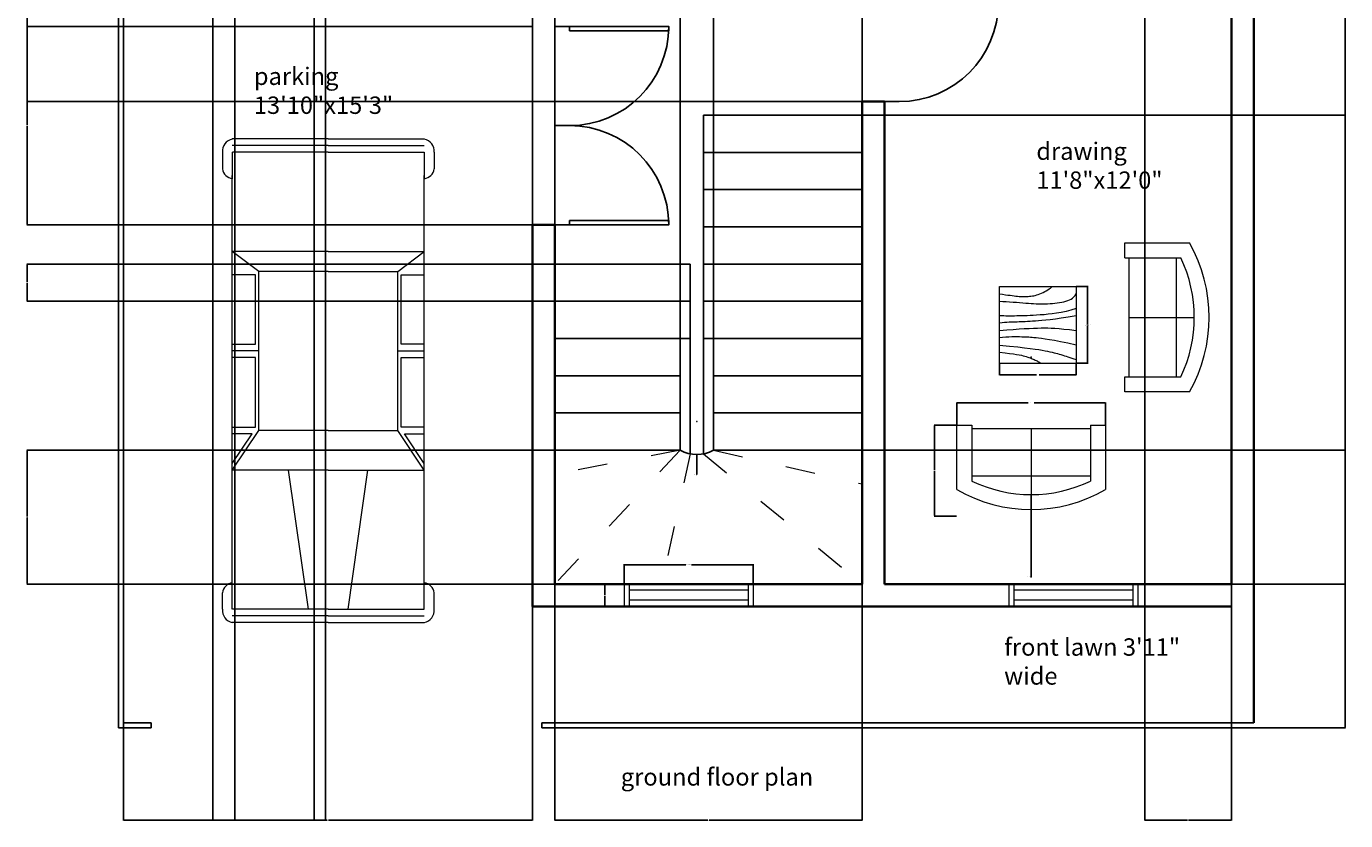
# Model space of a CAD drawing. Units: inches. Extents: x 1801 to 2333, y 478 to 1258.
# Tile 1 of 3: x 1801 to 2333, y 478 to 798. Entities that reach past the tile are written whole.
import ezdxf

# ---------------------------------------------------------------- set-up
doc = ezdxf.new("R2010")
doc.units = ezdxf.units.IN
doc.header["$MEASUREMENT"] = 0
doc.linetypes.add('ACAD_ISO03W100', pattern=[30, 12, -18])
for name, color, linetype, lineweight in [('A-ANNO-DIMS', 2, 'Continuous', 18), ('A-ANNO-TEXT', 7, 'Continuous', 25), ('A-AREA-IDEN', 7, 'Continuous', 18), ('A-DOOR', 4, 'Continuous', 25), ('A-FLOR-STRS', 7, 'Continuous', 25), ('A-FLOR-STRS-OVHD', 7, 'ACAD_ISO03W100', 18), ('A-FURN', 8, 'Continuous', 18), ('A-GLAZ', 4, 'Continuous', 18), ('A-WALL', 7, 'Continuous', 35), ('C-PKNG-VEHI', 8, 'Continuous', 13), ('C-PROP', 3, 'Continuous', 25)]:
    doc.layers.add(name, color=color, linetype=linetype, lineweight=lineweight)
doc.styles.get("Standard").update_dxf_attribs({"font": 'arial.ttf'})
doc.dimstyles.get("Standard").update_dxf_attribs({"dimtxt": 0.18, "dimasz": 0.18, "dimexe": 0.18, "dimexo": 0.0625, "dimgap": 0.09, "dimtad": 0, "dimtih": 1, "dimtoh": 1, "dimdec": 0, "dimzin": 0, "dimdsep": 46, "dimlunit": 3, "dimtxsty": 'Standard', "dimcen": 0.09, "dimadec": 0, "dimazin": 0, "dimtfac": 1, "dimtdec": 0, "dimtofl": 0, "dimtmove": 0, "dimatfit": 3, "dimfxl": 1, "dimtolj": 1, "dimtzin": 0, "dimarcsym": 0})

# ---------------------------------------------------------------- blocks, each defined once
blk = doc.blocks.new('*U2')
for p, q in [((0, 0), (0, -6)), ((40, 0), (40, -6))]:
    blk.add_line(p, q)
blk.add_lwpolyline([(0, 0), (0, 40), (1.75, 40), (1.75, 0)], close=True)
blk.add_arc((0, 0), 40, 0, 90)
blk = doc.blocks.new('*U4')
for p, q in [((0.1, -0.41), (0.1, 38.35)), ((2.77, -0.41), (2.77, 38.31)), ((5.44, 42.31), (12.12, 42.31)), ((5.44, -0.41), (5.44, 38.24)), ((5.45, 38.31), (16.12, 38.31)), ((16.12, 38.31), (180.34, 38.31)), ((61.52, -0.41), (61.52, 38.31)), ((61.52, 38.31), (77.54, 27.62)), ((64.19, 38.31), (76.2, 30.29)), ((76.2, 30.29), (76.2, 38.31)), ((78.87, 38.31), (78.87, 28.96)), ((106.91, 28.96), (106.91, 38.31)), ((109.58, 27.62), (109.58, 38.31)), ((112.25, 38.31), (112.25, 28.96)), ((140.29, 28.96), (140.29, 38.31)), ((141.62, 27.62), (149.64, 38.31)), ((149.64, -0.41), (149.64, 38.31)), ((189.69, 38.31), (179.01, 38.31)), ((189.69, 42.31), (183.01, 42.31)), ((189.69, -0.41), (189.69, 38.24)), ((192.36, -0.41), (192.36, 38.31)), ((195.03, -0.41), (195.03, 38.35)), ((77.54, 27.62), (141.62, 27.62)), ((77.54, -0.41), (77.54, 27.62)), ((78.87, 28.96), (106.91, 28.96)), ((112.25, 28.96), (140.29, 28.96)), ((141.62, -0.41), (141.62, 27.62)), ((5.44, 7.6), (61.52, 15.61)), ((0.1, -0.42), (0.1, -39.18)), ((2.77, -0.41), (2.77, -39.13)), ((5.44, -0.42), (5.44, -39.07)), ((61.52, -0.41), (61.52, -39.13)), ((77.54, -0.41), (77.54, -28.45)), ((141.62, -0.41), (141.62, -28.45)), ((149.64, -0.41), (149.64, -39.13)), ((189.69, -0.42), (189.69, -39.07)), ((192.36, -0.41), (192.36, -39.13)), ((195.03, -0.42), (195.03, -39.18)), ((5.44, -8.42), (61.52, -16.43)), ((61.52, -39.13), (77.54, -28.45)), ((64.19, -39.13), (76.2, -31.12)), ((76.2, -31.12), (76.2, -39.13)), ((77.54, -28.45), (141.62, -28.45)), ((78.87, -39.13), (78.87, -29.79)), ((78.87, -29.79), (106.91, -29.79)), ((106.91, -29.79), (106.91, -39.13)), ((109.58, -28.45), (109.58, -39.13)), ((112.25, -29.79), (140.29, -29.79)), ((112.25, -39.13), (112.25, -29.79)), ((140.29, -29.79), (140.29, -39.13)), ((141.62, -28.45), (149.64, -39.13)), ((5.45, -39.13), (16.12, -39.13)), ((16.12, -39.13), (180.34, -39.13)), ((189.69, -39.13), (179.01, -39.13)), ((5.44, -43.14), (12.12, -43.14)), ((189.69, -43.14), (183.01, -43.14))]:
    blk.add_line(p, q)
for centre, radius, start, end in [((5.06, 37.26), 5.06, 85.6455, 168.0943), ((11.45, 37.64), 4.72, 8.1301, 81.87), ((183.68, 37.64), 4.72, 98.13, 171.8699), ((190.07, 37.26), 5.06, 11.9057, 94.3545), ((5.06, -38.09), 5.06, 191.9057, 274.3545), ((11.45, -38.46), 4.72, 278.13, 351.8699), ((183.68, -38.46), 4.72, 188.1301, 261.87), ((190.07, -38.09), 5.06, 265.6455, 348.0943)]:
    blk.add_arc(centre, radius, start, end)
blk = doc.blocks.new('Sofa - Roundback Loveseat 5 ft.')
for p, q in [((0, -32.44198), (0, -5.99998)), ((-24, -33.99998), (-24, -11.46958)), ((-23.9998, -13.38178), (23.99986, -13.38178)), ((24.00004, -33.99998), (24.00004, -11.46958)), ((-24, -32.44198), (24.00004, -32.44198))]:
    blk.add_line(p, q)
for points in [[(-24, -33.99998), (-30, -33.99998), (-30, -7.99998)], [(30.00004, -7.99998), (30.00004, -33.99998), (24.00004, -33.99998)]]:
    blk.add_lwpolyline(points)
for centre, radius, start, end in [((0, -60.24998), 60.24998, 60.13715, 119.8628), ((0, -61.38438), 55.38444, 64.32083, 115.6792)]:
    blk.add_arc(centre, radius, start, end)
blk = doc.blocks.new('Table - Square Woodgrain 42 x 42 in.')
blk.add_line((0, -42), (42, -42))
for points in [[(0, -4), (1.704, -4.2172), (3.2358, -4.4188), (4.615, -4.604), (5.8615, -4.7721), (6.9951, -4.9224), (8.0357, -5.0541), (9.0031, -5.1667), (9.9171, -5.2594), (10.7951, -5.3316), (11.6445, -5.3836), (12.4702, -5.4157), (13.277, -5.4283), (14.0698, -5.4217), (14.8535, -5.3964), (15.6331, -5.3526), (16.4133, -5.2908), (17.1986, -5.2103), (17.9913, -5.1062), (18.793, -4.9727), (19.6056, -4.8038), (20.4307, -4.5937), (21.2701, -4.3365), (22.1256, -4.0262), (22.9989, -3.6571), (23.888, -3.2272), (24.7756, -2.7516), (25.6408, -2.2491), (26.4624, -1.7387), (27.2195, -1.2395), (27.891, -0.7703), (28.456, -0.3501), (28.8934, 0.002)], [(0, -42), (0, 0), (42, 0), (42, -42)], [(0, -8), (1.8203, -8.1001), (3.6741, -8.2149), (5.5411, -8.3408), (7.4011, -8.4741), (9.2339, -8.6112), (11.0193, -8.7484), (12.7371, -8.8821), (14.3671, -9.0086), (15.8954, -9.1246), (17.3337, -9.2278), (18.6997, -9.3159), (20.0116, -9.387), (21.2871, -9.4389), (22.5442, -9.4696), (23.8008, -9.477), (25.0749, -9.459), (26.3791, -9.4137), (27.7049, -9.3403), (29.0383, -9.2382), (30.3655, -9.1068), (31.6728, -8.9455), (32.9461, -8.7535), (34.1717, -8.5304), (35.3358, -8.2756), (36.4268, -7.9863), (37.443, -7.6521), (38.3849, -7.2603), (39.253, -6.7986), (40.048, -6.2542), (40.7705, -5.6147), (41.421, -4.8674), (42, -4)], [(42, -12), (39.1784, -12.8621), (36.4519, -13.5654), (33.8246, -14.1294), (31.3004, -14.5731), (28.8832, -14.9161), (26.577, -15.1775), (24.3858, -15.3768), (22.3136, -15.5332), (20.3622, -15.6632), (18.5254, -15.7718), (16.7947, -15.8612), (15.1618, -15.9338), (13.6183, -15.9916), (12.1558, -16.0369), (10.7659, -16.0718), (9.4403, -16.0987), (8.1703, -16.1191), (6.9461, -16.1325), (5.7577, -16.1377), (4.595, -16.1335), (3.4479, -16.1188), (2.3064, -16.0924), (1.1604, -16.0532), (0, -16)], [(42, -16), (37.6529, -16.7365), (33.8802, -17.329), (30.6179, -17.7961), (27.8015, -18.1561), (25.3668, -18.4275), (23.2497, -18.6288), (21.3859, -18.7785), (19.7111, -18.8949), (18.1693, -18.9939), (16.7375, -19.0795), (15.401, -19.1534), (14.1449, -19.217), (12.9544, -19.2717), (11.8148, -19.3191), (10.7113, -19.3606), (9.6291, -19.3976), (8.5534, -19.4323), (7.47, -19.4689), (6.3643, -19.5122), (5.222, -19.5672), (4.0288, -19.6386), (2.7703, -19.7313), (1.4321, -19.8501), (0, -20)], [(0, -24), (3.9243, -23.6805), (7.4766, -23.4138), (10.6891, -23.1954), (13.5943, -23.0205), (16.2247, -22.8847), (18.6125, -22.7832), (20.7903, -22.7116), (22.7903, -22.6651), (24.6563, -22.642), (26.4764, -22.6507), (28.35, -22.7024), (30.3766, -22.8084), (32.6555, -22.98), (35.2861, -23.2283), (38.3678, -23.5645), (42, -24)], [(42, -32), (37.392, -31.017), (33.4585, -30.2231), (30.1291, -29.5949), (27.3334, -29.109), (25.0009, -28.742), (23.0612, -28.4707), (21.4439, -28.2716), (20.0786, -28.1215), (18.8998, -28.0002), (17.8609, -27.9014), (16.9206, -27.8219), (16.0371, -27.7588), (15.1691, -27.709), (14.2748, -27.6693), (13.3128, -27.6368), (12.2415, -27.6083), (11.0295, -27.5824), (9.6867, -27.5643), (8.233, -27.5608), (6.6884, -27.5787), (5.0728, -27.6248), (3.4062, -27.7058), (1.7086, -27.8286), (0, -28)], [(0, -32), (5.4026, -32.5358), (9.9494, -33.019), (13.7424, -33.4553), (16.8834, -33.8505), (19.4743, -34.2106), (21.6171, -34.5413), (23.4136, -34.8486), (24.9657, -35.1382), (26.3614, -35.4156), (27.6332, -35.6841), (28.7995, -35.9467), (29.8788, -36.2064), (30.8897, -36.4661), (31.8507, -36.7288), (32.7802, -36.9973), (33.6968, -37.2747), (34.6175, -37.5635), (35.5531, -37.8651), (36.5128, -38.1805), (37.506, -38.5108), (38.5421, -38.8568), (39.6302, -39.2197), (40.7797, -39.6004), (42, -40)], [(0, -36), (3.0098, -36.2857), (5.5354, -36.5643), (7.6368, -36.8359), (9.374, -37.1009), (10.807, -37.3597), (11.9957, -37.6126), (13.0002, -37.8599), (13.8804, -38.102), (14.6874, -38.3393), (15.4365, -38.5729), (16.1338, -38.8041), (16.7858, -39.0341), (17.3987, -39.264), (17.9787, -39.4952), (18.5322, -39.7288), (19.0655, -39.9662), (19.5832, -40.2081), (20.0842, -40.4544), (20.5657, -40.7046), (21.0249, -40.9581), (21.459, -41.2144), (21.8653, -41.4731), (22.2409, -41.7335), (22.5831, -41.9951)]]:
    blk.add_lwpolyline(points)
blk = doc.blocks.new('WIN-48IN')
for p, q in [((0, 0), (0, 9)), ((2, 0), (2, 9)), ((2, 6.5), (50, 6.5)), ((50, 0), (50, 9)), ((52, 0), (52, 9)), ((2, 2.5), (50, 2.5))]:
    blk.add_line(p, q)
blk = doc.blocks.new('*D17')
at = {"layer": 'A-ANNO-DIMS', "color": 0, "lineweight": -2, "transparency": 16777216}
for p, q in [((2042.33, 573.54), (2042.33, 581.45)), ((2042.51, 581.27), (2067.21, 581.27)), ((2094.15, 581.27), (2069.45, 581.27)), ((2094.33, 573.54), (2094.33, 581.45))]:
    blk.add_line(p, q, dxfattribs=at)
at = {"layer": 'A-ANNO-DIMS', "color": 0, "transparency": 16777216}
for points in [[(2042.51, 581.3), (2042.51, 581.24), (2042.33, 581.27)], [(2094.15, 581.3), (2094.15, 581.24), (2094.33, 581.27)]]:
    blk.add_solid(points, dxfattribs=at)
at = {"layer": 'Defpoints', "color": 0, "transparency": 16777216}
for p in [(2042.33, 581.27), (2042.33, 573.47), (2094.33, 573.47)]:
    blk.add_point(p, dxfattribs=at)
at = {"layer": 'A-ANNO-DIMS', "color": 0, "transparency": 16777216, "insert": (2068.33, 581.27), "char_height": 0.18, "attachment_point": 5}
blk.add_mtext('\\A1;WINDOW 52 TYP.', dxfattribs=at)
blk = doc.blocks.new('*D18')
at = {"layer": 'A-ANNO-DIMS', "color": 0, "lineweight": -2, "transparency": 16777216}
for p, q in [((2042.27, 573.47), (2034.35, 573.47)), ((2034.53, 573.29), (2034.53, 569.16)), ((2042.27, 564.47), (2034.35, 564.47)), ((2034.53, 564.65), (2034.53, 568.79))]:
    blk.add_line(p, q, dxfattribs=at)
at = {"layer": 'A-ANNO-DIMS', "color": 0, "transparency": 16777216}
for points in [[(2034.5, 573.29), (2034.56, 573.29), (2034.53, 573.47)], [(2034.5, 564.65), (2034.56, 564.65), (2034.53, 564.47)]]:
    blk.add_solid(points, dxfattribs=at)
at = {"layer": 'Defpoints', "color": 0, "transparency": 16777216}
for p in [(2042.33, 573.47), (2034.53, 564.47), (2042.33, 564.47)]:
    blk.add_point(p, dxfattribs=at)
at = {"layer": 'A-ANNO-DIMS', "color": 0, "transparency": 16777216, "insert": (2034.53, 568.97), "char_height": 0.18, "attachment_point": 5}
blk.add_mtext('\\A1;9 TYP.', dxfattribs=at)
blk = doc.blocks.new('*D21')
at = {"layer": 'A-ANNO-DIMS', "color": 0, "lineweight": -2, "transparency": 16777216}
for p, q in [((2176.48, 637.6), (2176.48, 646.72)), ((2176.66, 646.54), (2205.26, 646.54)), ((2236.3, 646.54), (2207.71, 646.54)), ((2236.48, 637.6), (2236.48, 646.72))]:
    blk.add_line(p, q, dxfattribs=at)
at = {"layer": 'A-ANNO-DIMS', "color": 0, "transparency": 16777216}
for points in [[(2176.66, 646.57), (2176.66, 646.51), (2176.48, 646.54)], [(2236.3, 646.57), (2236.3, 646.51), (2236.48, 646.54)]]:
    blk.add_solid(points, dxfattribs=at)
at = {"layer": 'Defpoints', "color": 0, "transparency": 16777216}
for p in [(2176.48, 646.54), (2176.48, 637.54), (2236.48, 637.54)]:
    blk.add_point(p, dxfattribs=at)
at = {"layer": 'A-ANNO-DIMS', "color": 0, "transparency": 16777216, "insert": (2206.48, 646.54), "char_height": 0.18, "attachment_point": 5}
blk.add_mtext('\\A1;LOVESEAT 60 TYP.', dxfattribs=at)
blk = doc.blocks.new('*D22')
at = {"layer": 'A-ANNO-DIMS', "color": 0, "lineweight": -2, "transparency": 16777216}
for p, q in [((2176.42, 637.54), (2167.3, 637.54)), ((2167.48, 637.36), (2167.48, 619.39)), ((2167.48, 601.05), (2167.48, 619.03)), ((2176.42, 600.87), (2167.3, 600.87))]:
    blk.add_line(p, q, dxfattribs=at)
at = {"layer": 'A-ANNO-DIMS', "color": 0, "transparency": 16777216}
for points in [[(2167.45, 637.36), (2167.51, 637.36), (2167.48, 637.54)], [(2167.45, 601.05), (2167.51, 601.05), (2167.48, 600.87)]]:
    blk.add_solid(points, dxfattribs=at)
at = {"layer": 'Defpoints', "color": 0, "transparency": 16777216}
for p in [(2176.48, 637.54), (2167.48, 600.87), (2176.48, 600.87)]:
    blk.add_point(p, dxfattribs=at)
at = {"layer": 'A-ANNO-DIMS', "color": 0, "transparency": 16777216, "insert": (2167.48, 619.21), "char_height": 0.18, "attachment_point": 5}
blk.add_mtext('\\A1;37 TYP.', dxfattribs=at)
blk = doc.blocks.new('*D27')
at = {"layer": 'A-ANNO-DIMS', "color": 0, "lineweight": -2, "transparency": 16777216}
for p, q in [((2224.69, 693.39), (2229.45, 693.39)), ((2229.27, 693.21), (2229.27, 678.12)), ((2229.27, 662.66), (2229.27, 677.75)), ((2224.69, 662.48), (2229.45, 662.48))]:
    blk.add_line(p, q, dxfattribs=at)
at = {"layer": 'A-ANNO-DIMS', "color": 0, "transparency": 16777216}
for points in [[(2229.24, 693.21), (2229.3, 693.21), (2229.27, 693.39)], [(2229.24, 662.66), (2229.3, 662.66), (2229.27, 662.48)]]:
    blk.add_solid(points, dxfattribs=at)
at = {"layer": 'Defpoints', "color": 0, "transparency": 16777216}
for p in [(2224.63, 693.39), (2229.27, 693.39), (2224.63, 662.48)]:
    blk.add_point(p, dxfattribs=at)
at = {"layer": 'A-ANNO-DIMS', "color": 0, "transparency": 16777216, "insert": (2229.27, 677.93), "char_height": 0.18, "attachment_point": 5}
blk.add_mtext('\\A1;LOW TABLE 31 TYP.', dxfattribs=at)
blk = doc.blocks.new('*D28')
at = {"layer": 'A-ANNO-DIMS', "color": 0, "lineweight": -2, "transparency": 16777216}
for p, q in [((2193.72, 662.41), (2193.72, 657.66)), ((2224.63, 662.41), (2224.63, 657.66)), ((2193.9, 657.84), (2208.64, 657.84)), ((2224.45, 657.84), (2209.7, 657.84))]:
    blk.add_line(p, q, dxfattribs=at)
at = {"layer": 'A-ANNO-DIMS', "color": 0, "transparency": 16777216}
for points in [[(2193.9, 657.87), (2193.9, 657.81), (2193.72, 657.84)], [(2224.45, 657.87), (2224.45, 657.81), (2224.63, 657.84)]]:
    blk.add_solid(points, dxfattribs=at)
at = {"layer": 'Defpoints', "color": 0, "transparency": 16777216}
for p in [(2193.72, 662.48), (2224.63, 662.48), (2224.63, 657.84)]:
    blk.add_point(p, dxfattribs=at)
at = {"layer": 'A-ANNO-DIMS', "color": 0, "transparency": 16777216, "insert": (2209.17, 657.84), "char_height": 0.18, "attachment_point": 5}
blk.add_mtext('\\A1;31 TYP.', dxfattribs=at)
blk = doc.blocks.new('*D36')
at = {"layer": 'A-ANNO-DIMS', "color": 0, "lineweight": -2, "transparency": 16777216}
for p, q in [((2296.35, 1206.47), (2333.32, 1206.47)), ((2333.14, 1206.29), (2333.14, 861.16)), ((2333.14, 515.65), (2333.14, 860.79)), ((2296.35, 515.47), (2333.32, 515.47))]:
    blk.add_line(p, q, dxfattribs=at)
at = {"layer": 'A-ANNO-DIMS', "color": 0, "transparency": 16777216}
for points in [[(2333.11, 1206.29), (2333.17, 1206.29), (2333.14, 1206.47)], [(2333.11, 515.65), (2333.17, 515.65), (2333.14, 515.47)]]:
    blk.add_solid(points, dxfattribs=at)
at = {"layer": 'Defpoints', "color": 0, "transparency": 16777216}
for p in [(2296.29, 1206.47), (2333.14, 1206.47), (2296.29, 515.47)]:
    blk.add_point(p, dxfattribs=at)
at = {"layer": 'A-ANNO-DIMS', "color": 0, "transparency": 16777216, "insert": (2333.14, 860.97), "char_height": 0.18, "attachment_point": 5}
blk.add_mtext('\\A1;691', dxfattribs=at)
blk = doc.blocks.new('*D37')
at = {"layer": 'A-ANNO-DIMS', "color": 0, "lineweight": -2, "transparency": 16777216}
for p, q in [((1840.29, 804.41), (1840.29, 478.11)), ((2005.29, 804.41), (2005.29, 478.11)), ((1840.47, 478.29), (1922.51, 478.29)), ((2005.11, 478.29), (1923.07, 478.29))]:
    blk.add_line(p, q, dxfattribs=at)
at = {"layer": 'A-ANNO-DIMS', "color": 0, "transparency": 16777216}
for points in [[(1840.47, 478.32), (1840.47, 478.26), (1840.29, 478.29)], [(2005.11, 478.32), (2005.11, 478.26), (2005.29, 478.29)]]:
    blk.add_solid(points, dxfattribs=at)
at = {"layer": 'Defpoints', "color": 0, "transparency": 16777216}
for p in [(1840.29, 804.47), (2005.29, 804.47), (2005.29, 478.29)]:
    blk.add_point(p, dxfattribs=at)
at = {"layer": 'A-ANNO-DIMS', "color": 0, "transparency": 16777216, "insert": (1922.79, 478.29), "char_height": 0.18, "attachment_point": 5}
blk.add_mtext('\\A1;165', dxfattribs=at)
blk = doc.blocks.new('*D38')
at = {"layer": 'A-ANNO-DIMS', "color": 0, "lineweight": -2, "transparency": 16777216}
for p, q in [((2014.29, 573.41), (2014.29, 478.11)), ((2138.29, 573.41), (2138.29, 478.11)), ((2014.47, 478.29), (2076.01, 478.29)), ((2138.11, 478.29), (2076.57, 478.29))]:
    blk.add_line(p, q, dxfattribs=at)
at = {"layer": 'A-ANNO-DIMS', "color": 0, "transparency": 16777216}
for points in [[(2014.47, 478.32), (2014.47, 478.26), (2014.29, 478.29)], [(2138.11, 478.32), (2138.11, 478.26), (2138.29, 478.29)]]:
    blk.add_solid(points, dxfattribs=at)
at = {"layer": 'Defpoints', "color": 0, "transparency": 16777216}
for p in [(2014.29, 573.47), (2138.29, 573.47), (2138.29, 478.29)]:
    blk.add_point(p, dxfattribs=at)
at = {"layer": 'A-ANNO-DIMS', "color": 0, "transparency": 16777216, "insert": (2076.29, 478.29), "char_height": 0.18, "attachment_point": 5}
blk.add_mtext('\\A1;124', dxfattribs=at)
blk = doc.blocks.new('*D41')
at = {"layer": 'A-ANNO-DIMS', "color": 0, "lineweight": -2, "transparency": 16777216}
for p, q in [((2287.35, 810.47), (2333.32, 810.47)), ((2333.14, 810.29), (2333.14, 692.16)), ((2333.14, 573.65), (2333.14, 691.79)), ((2287.35, 573.47), (2333.32, 573.47))]:
    blk.add_line(p, q, dxfattribs=at)
at = {"layer": 'A-ANNO-DIMS', "color": 0, "transparency": 16777216}
for points in [[(2333.11, 810.29), (2333.17, 810.29), (2333.14, 810.47)], [(2333.11, 573.65), (2333.17, 573.65), (2333.14, 573.47)]]:
    blk.add_solid(points, dxfattribs=at)
at = {"layer": 'Defpoints', "color": 0, "transparency": 16777216}
for p in [(2287.29, 810.47), (2333.14, 810.47), (2287.29, 573.47)]:
    blk.add_point(p, dxfattribs=at)
at = {"layer": 'A-ANNO-DIMS', "color": 0, "transparency": 16777216, "insert": (2333.14, 691.97), "char_height": 0.18, "attachment_point": 5}
blk.add_mtext('\\A1;237', dxfattribs=at)
blk = doc.blocks.new('*D45')
at = {"layer": 'A-ANNO-DIMS', "color": 0, "lineweight": -2, "transparency": 16777216}
for p, q in [((1876.29, 1002.41), (1876.29, 478.11)), ((1917.2, 1002.41), (1917.2, 478.11)), ((1876.47, 478.29), (1896.36, 478.29)), ((1917.02, 478.29), (1897.12, 478.29))]:
    blk.add_line(p, q, dxfattribs=at)
at = {"layer": 'A-ANNO-DIMS', "color": 0, "transparency": 16777216}
for points in [[(1876.47, 478.32), (1876.47, 478.26), (1876.29, 478.29)], [(1917.02, 478.32), (1917.02, 478.26), (1917.2, 478.29)]]:
    blk.add_solid(points, dxfattribs=at)
at = {"layer": 'Defpoints', "color": 0, "transparency": 16777216}
for p in [(1876.29, 1002.47), (1917.2, 1002.47), (1917.2, 478.29)]:
    blk.add_point(p, dxfattribs=at)
at = {"layer": 'A-ANNO-DIMS', "color": 0, "transparency": 16777216, "insert": (1896.74, 478.29), "char_height": 0.18, "attachment_point": 5}
blk.add_mtext('\\A1;40.91', dxfattribs=at)
blk = doc.blocks.new('*D46')
at = {"layer": 'A-ANNO-DIMS', "color": 0, "lineweight": -2, "transparency": 16777216}
for p, q in [((2252.29, 963.41), (2252.29, 478.11)), ((2287.29, 963.41), (2287.29, 478.11)), ((2252.47, 478.29), (2269.57, 478.29)), ((2287.11, 478.29), (2270.01, 478.29))]:
    blk.add_line(p, q, dxfattribs=at)
at = {"layer": 'A-ANNO-DIMS', "color": 0, "transparency": 16777216}
for points in [[(2252.47, 478.32), (2252.47, 478.26), (2252.29, 478.29)], [(2287.11, 478.32), (2287.11, 478.26), (2287.29, 478.29)]]:
    blk.add_solid(points, dxfattribs=at)
at = {"layer": 'Defpoints', "color": 0, "transparency": 16777216}
for p in [(2252.29, 963.47), (2287.29, 963.47), (2287.29, 478.29)]:
    blk.add_point(p, dxfattribs=at)
at = {"layer": 'A-ANNO-DIMS', "color": 0, "transparency": 16777216, "insert": (2269.79, 478.29), "char_height": 0.18, "attachment_point": 5}
blk.add_mtext('\\A1;35', dxfattribs=at)
blk = doc.blocks.new('*D48')
at = {"layer": 'A-ANNO-DIMS', "color": 0, "lineweight": -2, "transparency": 16777216}
for p, q in [((2147.23, 810.47), (1801.26, 810.47)), ((1801.44, 810.29), (1801.44, 789.42)), ((1801.44, 768.17), (1801.44, 789.05)), ((2147.23, 767.99), (1801.26, 767.99))]:
    blk.add_line(p, q, dxfattribs=at)
at = {"layer": 'A-ANNO-DIMS', "color": 0, "transparency": 16777216}
for points in [[(1801.41, 810.29), (1801.47, 810.29), (1801.44, 810.47)], [(1801.41, 768.17), (1801.47, 768.17), (1801.44, 767.99)]]:
    blk.add_solid(points, dxfattribs=at)
at = {"layer": 'Defpoints', "color": 0, "transparency": 16777216}
for p in [(1801.44, 810.47), (2147.29, 810.47), (2147.29, 767.99)]:
    blk.add_point(p, dxfattribs=at)
at = {"layer": 'A-ANNO-DIMS', "color": 0, "transparency": 16777216, "insert": (1801.44, 789.23), "char_height": 0.18, "attachment_point": 5}
blk.add_mtext('\\A1;42.48', dxfattribs=at)
blk = doc.blocks.new('*D52')
at = {"layer": 'A-ANNO-DIMS', "color": 0, "lineweight": -2, "transparency": 16777216}
for p, q in [((1921.82, 814.91), (1921.82, 478.11)), ((1885.29, 813.41), (1885.29, 478.11)), ((1885.47, 478.29), (1903.09, 478.29)), ((1921.64, 478.29), (1904.02, 478.29))]:
    blk.add_line(p, q, dxfattribs=at)
at = {"layer": 'A-ANNO-DIMS', "color": 0, "transparency": 16777216}
for points in [[(1885.47, 478.32), (1885.47, 478.26), (1885.29, 478.29)], [(1921.64, 478.32), (1921.64, 478.26), (1921.82, 478.29)]]:
    blk.add_solid(points, dxfattribs=at)
at = {"layer": 'Defpoints', "color": 0, "transparency": 16777216}
for p in [(1921.82, 814.97), (1885.29, 813.47), (1921.82, 478.29)]:
    blk.add_point(p, dxfattribs=at)
at = {"layer": 'A-ANNO-DIMS', "color": 0, "transparency": 16777216, "insert": (1903.56, 478.29), "char_height": 0.18, "attachment_point": 5}
blk.add_mtext('\\A1;36.534', dxfattribs=at)
blk = doc.blocks.new('*D55')
at = {"layer": 'A-ANNO-DIMS', "color": 0, "lineweight": -2, "transparency": 16777216}
for p, q in [((2014.29, 702.54), (2014.29, 1257.55)), ((2014.47, 1257.37), (2039.21, 1257.37)), ((2064.75, 1257.37), (2040, 1257.37)), ((2064.93, 702.54), (2064.93, 1257.55))]:
    blk.add_line(p, q, dxfattribs=at)
at = {"layer": 'A-ANNO-DIMS', "color": 0, "transparency": 16777216}
for points in [[(2014.47, 1257.4), (2014.47, 1257.34), (2014.29, 1257.37)], [(2064.75, 1257.4), (2064.75, 1257.34), (2064.93, 1257.37)]]:
    blk.add_solid(points, dxfattribs=at)
at = {"layer": 'Defpoints', "color": 0, "transparency": 16777216}
for p in [(2064.93, 1257.37), (2014.29, 702.47), (2064.93, 702.47)]:
    blk.add_point(p, dxfattribs=at)
at = {"layer": 'A-ANNO-DIMS', "color": 0, "transparency": 16777216, "insert": (2039.61, 1257.37), "char_height": 0.18, "attachment_point": 5}
blk.add_mtext('\\A1;50.64', dxfattribs=at)
blk = doc.blocks.new('*D56')
at = {"layer": 'A-ANNO-DIMS', "color": 0, "lineweight": -2, "transparency": 16777216}
for p, q in [((2014.23, 702.47), (1801.26, 702.47)), ((1801.44, 702.29), (1801.44, 695.16)), ((1801.44, 687.65), (1801.44, 694.79)), ((2014.23, 687.47), (1801.26, 687.47))]:
    blk.add_line(p, q, dxfattribs=at)
at = {"layer": 'A-ANNO-DIMS', "color": 0, "transparency": 16777216}
for points in [[(1801.41, 702.29), (1801.47, 702.29), (1801.44, 702.47)], [(1801.41, 687.65), (1801.47, 687.65), (1801.44, 687.47)]]:
    blk.add_solid(points, dxfattribs=at)
at = {"layer": 'Defpoints', "color": 0, "transparency": 16777216}
for p in [(1801.44, 702.47), (2014.29, 702.47), (2014.29, 687.47)]:
    blk.add_point(p, dxfattribs=at)
at = {"layer": 'A-ANNO-DIMS', "color": 0, "transparency": 16777216, "insert": (1801.44, 694.97), "char_height": 0.18, "attachment_point": 5}
blk.add_mtext('\\A1;15', dxfattribs=at)
blk = doc.blocks.new('*D57')
at = {"layer": 'A-ANNO-DIMS', "color": 0, "lineweight": -2, "transparency": 16777216}
for p, q in [((2014.23, 627.47), (1801.26, 627.47)), ((1801.44, 627.29), (1801.44, 600.66)), ((1801.44, 573.65), (1801.44, 600.29)), ((2014.23, 573.47), (1801.26, 573.47))]:
    blk.add_line(p, q, dxfattribs=at)
at = {"layer": 'A-ANNO-DIMS', "color": 0, "transparency": 16777216}
for points in [[(1801.41, 627.29), (1801.47, 627.29), (1801.44, 627.47)], [(1801.41, 573.65), (1801.47, 573.65), (1801.44, 573.47)]]:
    blk.add_solid(points, dxfattribs=at)
at = {"layer": 'Defpoints', "color": 0, "transparency": 16777216}
for p in [(1801.44, 627.47), (2014.29, 627.47), (2014.29, 573.47)]:
    blk.add_point(p, dxfattribs=at)
at = {"layer": 'A-ANNO-DIMS', "color": 0, "transparency": 16777216, "insert": (1801.44, 600.47), "char_height": 0.18, "attachment_point": 5}
blk.add_mtext('\\A1;54', dxfattribs=at)
blk = doc.blocks.new('*D58')
at = {"layer": 'A-ANNO-DIMS', "color": 0, "lineweight": -2, "transparency": 16777216}
for p, q in [((2138.35, 762.47), (2333.32, 762.47)), ((2333.14, 762.29), (2333.14, 695.16)), ((2333.14, 627.65), (2333.14, 694.79)), ((2138.35, 627.47), (2333.32, 627.47))]:
    blk.add_line(p, q, dxfattribs=at)
at = {"layer": 'A-ANNO-DIMS', "color": 0, "transparency": 16777216}
for points in [[(2333.11, 762.29), (2333.17, 762.29), (2333.14, 762.47)], [(2333.11, 627.65), (2333.17, 627.65), (2333.14, 627.47)]]:
    blk.add_solid(points, dxfattribs=at)
at = {"layer": 'Defpoints', "color": 0, "transparency": 16777216}
for p in [(2138.29, 762.47), (2333.14, 762.47), (2138.29, 627.47)]:
    blk.add_point(p, dxfattribs=at)
at = {"layer": 'A-ANNO-DIMS', "color": 0, "transparency": 16777216, "insert": (2333.14, 694.97), "char_height": 0.18, "attachment_point": 5}
blk.add_mtext('\\A1;135', dxfattribs=at)
blk = doc.blocks.new('*D59')
at = {"layer": 'A-ANNO-DIMS', "color": 0, "lineweight": -2, "transparency": 16777216}
for p, q in [((2078.29, 762.54), (2078.29, 1257.55)), ((2078.47, 1257.37), (2108.07, 1257.37)), ((2138.11, 1257.37), (2108.51, 1257.37)), ((2138.29, 762.54), (2138.29, 1257.55))]:
    blk.add_line(p, q, dxfattribs=at)
at = {"layer": 'A-ANNO-DIMS', "color": 0, "transparency": 16777216}
for points in [[(2078.47, 1257.4), (2078.47, 1257.34), (2078.29, 1257.37)], [(2138.11, 1257.4), (2138.11, 1257.34), (2138.29, 1257.37)]]:
    blk.add_solid(points, dxfattribs=at)
at = {"layer": 'Defpoints', "color": 0, "transparency": 16777216}
for p in [(2138.29, 1257.37), (2078.29, 762.47), (2138.29, 762.47)]:
    blk.add_point(p, dxfattribs=at)
at = {"layer": 'A-ANNO-DIMS', "color": 0, "transparency": 16777216, "insert": (2108.29, 1257.37), "char_height": 0.18, "attachment_point": 5}
blk.add_mtext('\\A1;60', dxfattribs=at)
blk = doc.blocks.new('*D60')
at = {"layer": 'A-ANNO-DIMS', "color": 0, "lineweight": -2, "transparency": 16777216}
for p, q in [((2005.23, 798.28), (1801.26, 798.28)), ((1801.44, 798.1), (1801.44, 758.47)), ((1801.44, 718.46), (1801.44, 758.1)), ((2005.23, 718.28), (1801.26, 718.28))]:
    blk.add_line(p, q, dxfattribs=at)
at = {"layer": 'A-ANNO-DIMS', "color": 0, "transparency": 16777216}
for points in [[(1801.41, 798.1), (1801.47, 798.1), (1801.44, 798.28)], [(1801.41, 718.46), (1801.47, 718.46), (1801.44, 718.28)]]:
    blk.add_solid(points, dxfattribs=at)
at = {"layer": 'Defpoints', "color": 0, "transparency": 16777216}
for p in [(1801.44, 798.28), (2005.29, 798.28), (2005.29, 718.28)]:
    blk.add_point(p, dxfattribs=at)
at = {"layer": 'A-ANNO-DIMS', "color": 0, "transparency": 16777216, "insert": (1801.44, 758.28), "char_height": 0.18, "attachment_point": 5}
blk.add_mtext('\\A1;80', dxfattribs=at)
blk = doc.blocks.new('*D62')
at = {"layer": 'A-ANNO-DIMS', "color": 0, "lineweight": -2, "transparency": 16777216}
for p, q in [((2206.39, 664.93), (2206.57, 664.93)), ((2206.48, 664.84), (2206.48, 665.02)), ((2206.48, 576.31), (2206.48, 609.36)), ((2206.3, 576.31), (2206.48, 576.31))]:
    blk.add_line(p, q, dxfattribs=at)
at = {"layer": 'A-ANNO-DIMS', "color": 0, "transparency": 16777216}
blk.add_solid([(2206.45, 609.36), (2206.51, 609.36), (2206.48, 609.54)], dxfattribs=at)
at = {"layer": 'Defpoints', "color": 0, "transparency": 16777216}
for p in [(2206.48, 664.93), (2206.48, 609.54)]:
    blk.add_point(p, dxfattribs=at)
at = {"layer": 'A-ANNO-DIMS', "color": 0, "transparency": 16777216, "insert": (2205.62, 576.31), "char_height": 0.18, "attachment_point": 5}
blk.add_mtext('\\A1;5X R55.38', dxfattribs=at)
blk = doc.blocks.new('*D63')
at = {"layer": 'A-ANNO-DIMS', "color": 0, "lineweight": -2, "transparency": 16777216}
for p, q in [((2071.52, 639.04), (2071.7, 639.04)), ((2071.61, 638.95), (2071.61, 639.13)), ((2071.61, 617.67), (2071.61, 625.5)), ((2071.43, 617.67), (2071.61, 617.67))]:
    blk.add_line(p, q, dxfattribs=at)
at = {"layer": 'A-ANNO-DIMS', "color": 0, "transparency": 16777216}
blk.add_solid([(2071.58, 625.5), (2071.64, 625.5), (2071.61, 625.68)], dxfattribs=at)
at = {"layer": 'Defpoints', "color": 0, "transparency": 16777216}
for p in [(2071.61, 639.04), (2071.61, 625.68)]:
    blk.add_point(p, dxfattribs=at)
at = {"layer": 'A-ANNO-DIMS', "color": 0, "transparency": 16777216, "insert": (2070.88, 617.67), "char_height": 0.18, "attachment_point": 5}
blk.add_mtext('\\A1;R13.357', dxfattribs=at)

msp = doc.modelspace()

# ---------------------------------------------------------------- linework, layer by layer
at = {"layer": 'A-FLOR-STRS'}
for p, q in [((2138.2881, 762.4747), (2074.2881, 762.4747)), ((2074.2881, 625.9557), (2074.2881, 762.4747)), ((2078.2881, 627.4747), (2078.2881, 762.4747)), ((2138.2881, 747.4747), (2074.2881, 747.4747)), ((2138.2881, 732.4747), (2074.2881, 732.4747)), ((2138.2881, 717.4747), (2074.2881, 717.4747)), ((2068.9263, 702.4747), (2014.2881, 702.4747)), ((2064.9263, 627.4747), (2064.9263, 702.4747)), ((2068.9263, 625.9557), (2068.9263, 702.4747)), ((2138.2881, 702.4747), (2074.2881, 702.4747)), ((2068.9263, 687.4747), (2014.2881, 687.4747)), ((2138.2881, 687.4747), (2074.2881, 687.4747)), ((2068.9263, 672.4747), (2014.2881, 672.4747)), ((2138.2881, 672.4747), (2074.2881, 672.4747)), ((2064.9263, 657.4747), (2014.2881, 657.4747)), ((2138.2881, 657.4747), (2078.2881, 657.4747)), ((2064.9263, 642.4747), (2014.2881, 642.4747)), ((2138.2881, 642.4747), (2078.2881, 642.4747)), ((2064.9263, 627.4747), (2014.2881, 627.4747)), ((2138.2881, 627.4747), (2078.2881, 627.4747))]:
    msp.add_line(p, q, dxfattribs=at)
msp.add_arc((2071.6072, 639.0411), 13.3572, 239.988561, 300.011439, dxfattribs=at)
at = {"layer": 'A-FLOR-STRS-OVHD'}
for p, q in [((2064.9263, 627.4747), (2014.2881, 617.7483)), ((2064.9263, 627.4747), (2014.2881, 573.4747)), ((2068.9263, 625.9557), (2057.3835, 573.4747)), ((2074.2881, 625.9557), (2138.2881, 573.4747)), ((2078.2881, 627.4747), (2138.2881, 613.8185))]:
    msp.add_line(p, q, dxfattribs=at)
at = {"layer": 'A-WALL'}
for p, q in [((2296.2881, 1206.4747), (2296.2881, 517.4747)), ((2287.2881, 810.4747), (2287.2881, 573.4747)), ((2138.2881, 767.9929), (2138.2881, 573.4747)), ((2147.2881, 767.9929), (2138.2881, 767.9929)), ((2147.2881, 767.9929), (2147.2881, 573.4747)), ((2014.2881, 718.2841), (2005.2881, 718.2841)), ((2005.2881, 718.2841), (2005.2881, 564.4747)), ((2014.2881, 718.2841), (2014.2881, 573.4747)), ((2138.2881, 573.4747), (2014.2881, 573.4747)), ((2287.2881, 573.4747), (2147.2881, 573.4747)), ((2287.2881, 564.4747), (2005.2881, 564.4747))]:
    msp.add_line(p, q, dxfattribs=at)
at = {"layer": 'C-PROP'}
for p, q in [((1838.2881, 515.4747), (1838.2881, 930.4747)), ((1840.2881, 517.4747), (1840.2881, 930.4747)), ((2287.2881, 564.4747), (2287.2881, 517.4747)), ((1851.5334, 517.4747), (1840.2881, 517.4747)), ((1851.5334, 517.4747), (1851.5334, 515.4747)), ((2296.2881, 517.4747), (2009.0818, 517.4747)), ((2009.0818, 517.4747), (2009.0818, 515.4747)), ((1851.5334, 515.4747), (1838.2881, 515.4747)), ((2296.2881, 515.4747), (2009.0818, 515.4747))]:
    msp.add_line(p, q, dxfattribs=at)

# ---------------------------------------------------------------- block references
at = {"layer": 'A-DOOR', "rotation": 270}
for p in [(2153.2881, 807.9929), (2020.2881, 798.2841)]:
    msp.add_blockref('*U2', p, dxfattribs=at)
at = {"layer": 'A-DOOR', "xscale": -1, "rotation": 270}
msp.add_blockref('*U2', (2020.2881, 718.2841), dxfattribs=at)
at = {"layer": 'A-FURN'}
for p, rotation in [((2278.3101, 680.9905), 270), ((2206.484, 603.5407), 180)]:
    msp.add_blockref('Sofa - Roundback Loveseat 5 ft.', p, dxfattribs=dict(at, rotation=rotation))
at = {"layer": 'A-FURN', "xscale": 0.7359782021052613, "yscale": 0.7359782021052613, "zscale": 0.7359782021052613}
msp.add_blockref('Table - Square Woodgrain 42 x 42 in.', (2193.7172, 693.387), dxfattribs=at)
at = {"layer": 'A-GLAZ', "rotation": 180}
for p in [(2094.3304, 573.4745), (2249.5236, 573.4745)]:
    msp.add_blockref('WIN-48IN', p, dxfattribs=at)
at = {"layer": 'C-PKNG-VEHI', "rotation": 90}
msp.add_blockref('*U4', (1922.5067, 557.8683), dxfattribs=at)

# ---------------------------------------------------------------- texts
at = {"layer": 'A-ANNO-TEXT', "insert": (2040.9406, 499.2277), "char_height": 7, "attachment_point": 1}
msp.add_mtext_dynamic_manual_height_columns('ground floor plan', width=376.152437, gutter_width=1, heights=[0], dxfattribs=at)
at = {"layer": 'A-AREA-IDEN', "char_height": 7, "attachment_point": 1}
for s, width, insert in [('parking\\P13\'10"x15\'3"\\P  ', 106.765691, (1892.9078, 781.6794)), ('drawing\\P11\'8"x12\'0"\\P  ', 106.765691, (2208.5683, 751.4845)), ('front lawn 3\'11" wide', 84.800625, (2195.6056, 551.5903))]:
    msp.add_mtext_dynamic_manual_height_columns(s, width=width, gutter_width=1, heights=[0], dxfattribs=dict(at, insert=insert))

# ---------------------------------------------------------------- dimensions: what is measured, and where the dimension line sits
at = {"layer": 'A-ANNO-DIMS'}
for base, p1, p2, override, picture, middle in [((2064.9263, 1257.3702), (2014.2881, 702.4747), (2064.9263, 702.4747), {"dimdec": 2, "dimlfac": 1, "dimrnd": 0, "dimzin": 0, "dimdsep": 46, "dimlunit": 2}, '*D55', (2039.6072, 1257.3702)), ((2138.2881, 1257.3702), (2078.2881, 762.4747), (2138.2881, 762.4747), {"dimdec": 0, "dimlfac": 1, "dimrnd": 0, "dimzin": 0, "dimdsep": 46, "dimlunit": 2}, '*D59', (2108.2881, 1257.3702)), ((1917.1982, 478.2946), (1876.2881, 1002.4747), (1917.1982, 1002.4747), {"dimdec": 2, "dimlfac": 1, "dimrnd": 0, "dimzin": 0, "dimdsep": 46, "dimlunit": 2}, '*D45', (1896.7431, 478.2946)), ((2287.2881, 478.2946), (2252.2853, 963.4747), (2287.2881, 963.4747), {"dimdec": 0, "dimlfac": 1, "dimrnd": 0, "dimzin": 0, "dimdsep": 46, "dimlunit": 2}, '*D46', (2269.7867, 478.2946)), ((1921.8221, 478.2946), (1885.2881, 813.4747), (1921.8221, 814.9737), {"dimdec": 3, "dimlfac": 1, "dimrnd": 0, "dimzin": 0, "dimdsep": 46, "dimlunit": 2}, '*D52', (1903.5551, 478.2946)), ((2005.2881, 478.2946), (1840.2881, 804.4747), (2005.2881, 804.4747), {"dimdec": 0, "dimlfac": 1, "dimrnd": 0, "dimzin": 0, "dimdsep": 46, "dimlunit": 2}, '*D37', (1922.7881, 478.2946)), ((2138.2881, 478.2946), (2014.2881, 573.4747), (2138.2881, 573.4747), {"dimdec": 0, "dimlfac": 1, "dimrnd": 0, "dimzin": 0, "dimdsep": 46, "dimlunit": 2}, '*D38', (2076.2881, 478.2946))]:
    dim = msp.add_linear_dim(base=base, p1=p1, p2=p2, dimstyle='Standard', override=override, dxfattribs=at)
    dim.commit()
    dim.dimension.update_dxf_attribs({"geometry": picture, "text_midpoint": middle})
for base, p1, p2, override, picture, middle in [((2333.1381, 1206.4747), (2296.2881, 515.4747), (2296.2881, 1206.4747), {"dimdec": 0, "dimlfac": 1, "dimrnd": 0, "dimzin": 0, "dimdsep": 46, "dimlunit": 2}, '*D36', (2333.1381, 860.9747)), ((1801.4381, 810.4747), (2147.2881, 767.9929), (2147.2881, 810.4747), {"dimdec": 2, "dimlfac": 1, "dimrnd": 0, "dimzin": 0, "dimdsep": 46, "dimlunit": 2}, '*D48', (1801.4381, 789.2338)), ((2333.1381, 810.4747), (2287.2881, 573.4747), (2287.2881, 810.4747), {"dimdec": 0, "dimlfac": 1, "dimrnd": 0, "dimzin": 0, "dimdsep": 46, "dimlunit": 2}, '*D41', (2333.1381, 691.9747)), ((1801.4381, 798.2841), (2005.2881, 718.2841), (2005.2881, 798.2841), {"dimdec": 0, "dimlfac": 1, "dimrnd": 0, "dimzin": 0, "dimdsep": 46, "dimlunit": 2}, '*D60', (1801.4381, 758.2841)), ((2333.1381, 762.4747), (2138.2881, 627.4747), (2138.2881, 762.4747), {"dimdec": 0, "dimlfac": 1, "dimrnd": 0, "dimzin": 0, "dimdsep": 46, "dimlunit": 2}, '*D58', (2333.1381, 694.9747)), ((1801.4381, 702.4747), (2014.2881, 687.4747), (2014.2881, 702.4747), {"dimdec": 0, "dimlfac": 1, "dimrnd": 0, "dimzin": 0, "dimdsep": 46, "dimlunit": 2}, '*D56', (1801.4381, 694.9747)), ((1801.4381, 627.4747), (2014.2881, 573.4747), (2014.2881, 627.4747), {"dimdec": 0, "dimlfac": 1, "dimrnd": 0, "dimzin": 0, "dimdsep": 46, "dimlunit": 2}, '*D57', (1801.4381, 600.4747))]:
    dim = msp.add_linear_dim(base=base, p1=p1, p2=p2, angle=90, dimstyle='Standard', override=override, dxfattribs=at)
    dim.commit()
    dim.dimension.update_dxf_attribs({"geometry": picture, "text_midpoint": middle})
for base, p1, p2, angle, text, picture, middle in [((2229.2651, 693.3885), (2224.6282, 662.4759), (2224.6282, 693.3885), 90, 'LOW TABLE <> TYP.', '*D27', (2229.2651, 677.9322)), ((2176.4839, 646.5407), (2236.484, 637.5407), (2176.4839, 637.5407), 180, 'LOVESEAT <> TYP.', '*D21', (2206.484, 646.5407)), ((2167.4839, 600.8741), (2176.4839, 637.5407), (2176.4839, 600.8741), 270, '<> TYP.', '*D22', (2167.4839, 619.2074)), ((2042.3303, 581.2747), (2094.3303, 573.4747), (2042.3303, 573.4747), 180, 'WINDOW <> TYP.', '*D17', (2068.3303, 581.2747)), ((2034.5303, 564.4747), (2042.3303, 573.4747), (2042.3303, 564.4747), 270, '<> TYP.', '*D18', (2034.5303, 568.9747))]:
    dim = msp.add_linear_dim(base=base, p1=p1, p2=p2, angle=angle, text=text, dimstyle='Standard', override={"dimdec": 0, "dimlfac": 1, "dimrnd": 0, "dimzin": 0, "dimdsep": 46, "dimlunit": 2}, dxfattribs=at)
    dim.commit()
    dim.dimension.update_dxf_attribs({"geometry": picture, "text_midpoint": middle})
dim = msp.add_linear_dim(base=(2224.6282, 657.8391), p1=(2193.7172, 662.4759), p2=(2224.6282, 662.4759), text='<> TYP.', dimstyle='Standard', override={"dimdec": 0, "dimlfac": 1, "dimrnd": 0, "dimzin": 0, "dimdsep": 46, "dimlunit": 2}, dxfattribs=at)
dim.commit()
dim.dimension.update_dxf_attribs({"geometry": '*D28', "text_midpoint": (2209.1727, 657.8391)})
dim = msp.add_radius_dim(center=(2206.484, 664.9251), mpoint=(2206.48, 609.5407), text='5X <>', dimstyle='Standard', override={"dimdec": 2, "dimlfac": 1, "dimrnd": 0, "dimzin": 0, "dimdsep": 46, "dimlunit": 2}, dxfattribs=at)
dim.commit()
dim.dimension.update_dxf_attribs({"geometry": '*D62', "text_midpoint": (2205.6242, 576.31), "dimtype": 164})
dim = msp.add_radius_dim(center=(2071.6072, 639.0411), mpoint=(2071.607, 625.6839), dimstyle='Standard', override={"dimdec": 3, "dimlfac": 1, "dimrnd": 0, "dimzin": 0, "dimdsep": 46, "dimlunit": 2}, dxfattribs=at)
dim.commit()
dim.dimension.update_dxf_attribs({"geometry": '*D63', "text_midpoint": (2070.8771, 617.6696), "dimtype": 164})

doc.saveas('drawing.dxf')
